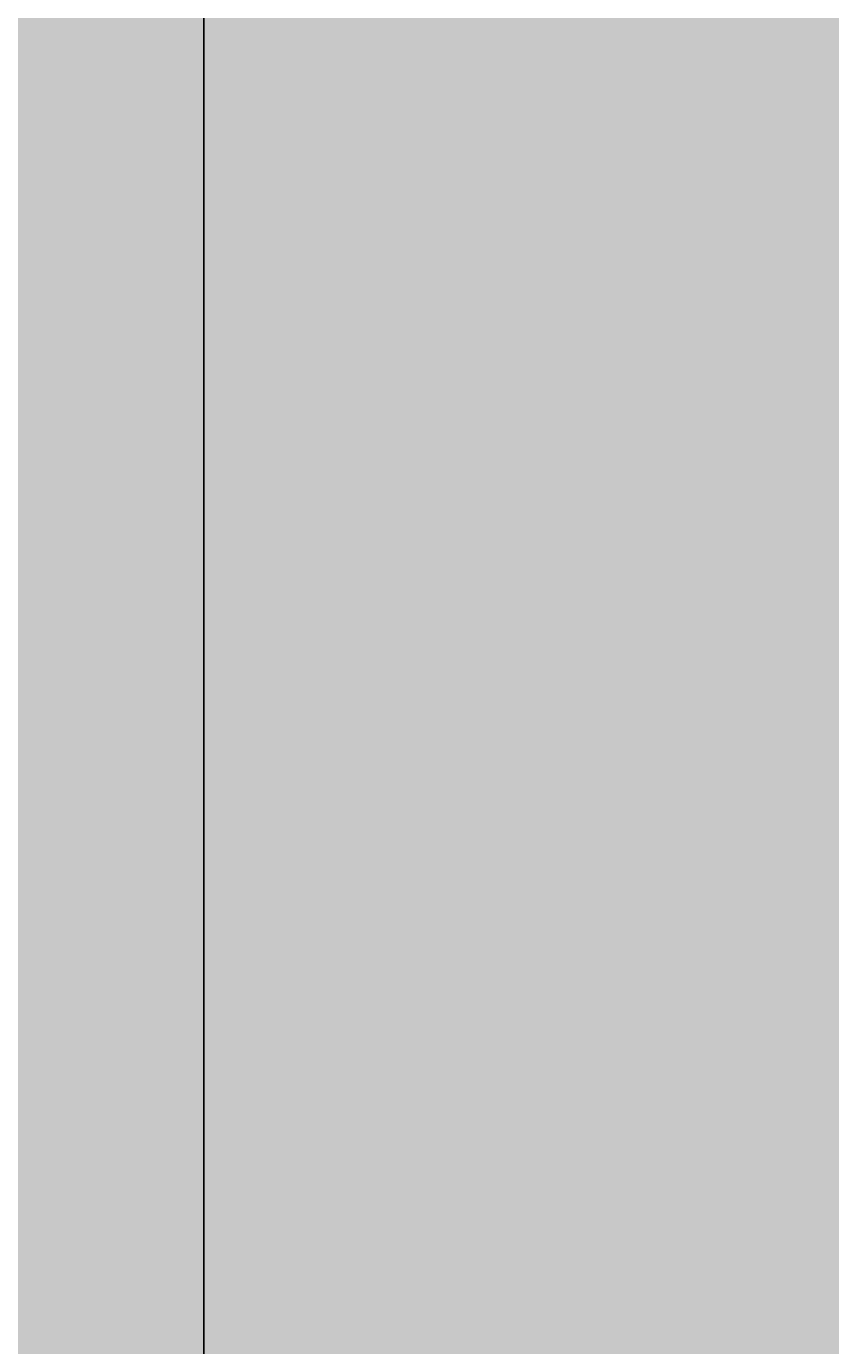
# Model space of a CAD drawing. Units: millimetres. Extents: x -22994 to 29398, y -19990 to 20176.
# Tile 105 of 135: x 198 to 216, y 95 to 124. Entities that reach past the tile are written whole.
import ezdxf

# ---------------------------------------------------------------- set-up
doc = ezdxf.new("R2010")
doc.units = ezdxf.units.MM
doc.header["$MEASUREMENT"] = 0
for name, color, linetype, lineweight in [('M-DIMS', 2, 'Continuous', 18), ('M-EQPM', 7, 'Continuous', 25), ('M-EQPM-PATT', 7, 'Continuous', 18)]:
    doc.layers.add(name, color=color, linetype=linetype, lineweight=lineweight)
doc.styles.get("Standard").update_dxf_attribs({"font": 'arial.ttf'})
doc.dimstyles.get("Standard").update_dxf_attribs({"dimtxt": 0.18, "dimasz": 10000, "dimexe": 0.18, "dimexo": 0.0625, "dimgap": 0.09, "dimtad": 0, "dimtih": 1, "dimtoh": 1, "dimdec": 0, "dimzin": 0, "dimdsep": 46, "dimtxsty": 'Standard', "dimcen": 0.09, "dimadec": 0, "dimazin": 0, "dimtfac": 1, "dimtdec": 0, "dimtofl": 0, "dimtmove": 0, "dimatfit": 3, "dimfxl": 1, "dimtolj": 1, "dimtzin": 0, "dimlwd": 30, "dimarcsym": 0})

# ---------------------------------------------------------------- blocks, each defined once
blk = doc.blocks.new('*D2')
at = {"layer": 'Defpoints', "color": 0, "transparency": 16777216}
for p in [(6.677, 10.271), (290.852, 10.271), (290.852, -5.079)]:
    blk.add_point(p, dxfattribs=at)
at = {"layer": 'M-DIMS', "color": 0, "lineweight": -2, "transparency": 16777216}
for p, q in [((6.677, 10.209), (6.677, -5.259)), ((290.852, 10.209), (290.852, -5.259))]:
    blk.add_line(p, q, dxfattribs=at)
at = {"layer": 'M-DIMS', "color": 0, "lineweight": 30, "transparency": 16777216}
for p, q in [((-9993.323, -5.079), (-19993.323, -5.079)), ((10290.852, -5.079), (20290.852, -5.079))]:
    blk.add_line(p, q, dxfattribs=at)
at = {"layer": 'M-DIMS', "color": 0, "transparency": 16777216}
for points in [[(-9993.323, 1661.588), (-9993.323, -1671.745), (6.677, -5.079)], [(10290.852, 1661.588), (10290.852, -1671.745), (290.852, -5.079)]]:
    blk.add_solid(points, dxfattribs=at)
at = {"layer": 'M-DIMS', "color": 0, "transparency": 16777216, "insert": (148.765, -5.079), "char_height": 0.18, "attachment_point": 5}
blk.add_mtext('\\A1;284.2', dxfattribs=at)
blk = doc.blocks.new('*D3')
at = {"layer": 'Defpoints', "color": 0, "transparency": 16777216}
for p in [(110.265, 204.165), (110.265, 176.366), (95.833, 127.967)]:
    blk.add_point(p, dxfattribs=at)
at = {"layer": 'M-DIMS', "color": 0, "lineweight": -2, "transparency": 16777216}
for p, q in [((95.833, 128.03), (95.833, 204.345)), ((110.265, 176.429), (110.265, 204.345))]:
    blk.add_line(p, q, dxfattribs=at)
at = {"layer": 'M-DIMS', "color": 0, "lineweight": 30, "transparency": 16777216}
for p, q in [((-9904.167, 204.165), (-19904.167, 204.165)), ((10110.265, 204.165), (20110.265, 204.165))]:
    blk.add_line(p, q, dxfattribs=at)
at = {"layer": 'M-DIMS', "color": 0, "transparency": 16777216}
for points in [[(-9904.167, 1870.832), (-9904.167, -1462.501), (95.833, 204.165)], [(10110.265, 1870.832), (10110.265, -1462.501), (110.265, 204.165)]]:
    blk.add_solid(points, dxfattribs=at)
at = {"layer": 'M-DIMS', "color": 0, "transparency": 16777216, "insert": (103.049, 204.165), "char_height": 0.18, "attachment_point": 5}
blk.add_mtext('\\A1;14.432', dxfattribs=at)
blk = doc.blocks.new('*D4')
at = {"layer": 'Defpoints', "color": 0, "transparency": 16777216}
for p in [(116.265, 204.165), (110.265, 176.366), (116.265, 176.366)]:
    blk.add_point(p, dxfattribs=at)
at = {"layer": 'M-DIMS', "color": 0, "lineweight": -2, "transparency": 16777216}
for p, q in [((110.265, 176.429), (110.265, 204.345)), ((116.265, 176.429), (116.265, 204.345))]:
    blk.add_line(p, q, dxfattribs=at)
at = {"layer": 'M-DIMS', "color": 0, "lineweight": 30, "transparency": 16777216}
for p, q in [((-9889.735, 204.165), (-19889.735, 204.165)), ((10116.265, 204.165), (20116.265, 204.165))]:
    blk.add_line(p, q, dxfattribs=at)
at = {"layer": 'M-DIMS', "color": 0, "transparency": 16777216}
for points in [[(-9889.735, 1870.832), (-9889.735, -1462.501), (110.265, 204.165)], [(10116.265, 1870.832), (10116.265, -1462.501), (116.265, 204.165)]]:
    blk.add_solid(points, dxfattribs=at)
at = {"layer": 'M-DIMS', "color": 0, "transparency": 16777216, "insert": (113.265, 204.165), "char_height": 0.18, "attachment_point": 5}
blk.add_mtext('\\A1;6', dxfattribs=at)
blk = doc.blocks.new('*D5')
at = {"layer": 'Defpoints', "color": 0, "transparency": 16777216}
for p in [(181.265, 204.165), (116.265, 176.366), (181.265, 176.366)]:
    blk.add_point(p, dxfattribs=at)
at = {"layer": 'M-DIMS', "color": 0, "lineweight": -2, "transparency": 16777216}
for p, q in [((116.265, 176.429), (116.265, 204.345)), ((181.265, 176.429), (181.265, 204.345))]:
    blk.add_line(p, q, dxfattribs=at)
at = {"layer": 'M-DIMS', "color": 0, "lineweight": 30, "transparency": 16777216}
for p, q in [((-9883.735, 204.165), (-19883.735, 204.165)), ((10181.265, 204.165), (20181.265, 204.165))]:
    blk.add_line(p, q, dxfattribs=at)
at = {"layer": 'M-DIMS', "color": 0, "transparency": 16777216}
for points in [[(-9883.735, 1870.832), (-9883.735, -1462.501), (116.265, 204.165)], [(10181.265, 1870.832), (10181.265, -1462.501), (181.265, 204.165)]]:
    blk.add_solid(points, dxfattribs=at)
at = {"layer": 'M-DIMS', "color": 0, "transparency": 16777216, "insert": (148.765, 204.165), "char_height": 0.18, "attachment_point": 5}
blk.add_mtext('\\A1;65', dxfattribs=at)
blk = doc.blocks.new('*D6')
at = {"layer": 'Defpoints', "color": 0, "transparency": 16777216}
for p in [(187.265, 204.165), (181.265, 176.366), (187.265, 176.366)]:
    blk.add_point(p, dxfattribs=at)
at = {"layer": 'M-DIMS', "color": 0, "lineweight": -2, "transparency": 16777216}
for p, q in [((181.265, 176.429), (181.265, 204.345)), ((187.265, 176.429), (187.265, 204.345))]:
    blk.add_line(p, q, dxfattribs=at)
at = {"layer": 'M-DIMS', "color": 0, "lineweight": 30, "transparency": 16777216}
for p, q in [((-9818.735, 204.165), (-19818.735, 204.165)), ((10187.265, 204.165), (20187.265, 204.165))]:
    blk.add_line(p, q, dxfattribs=at)
at = {"layer": 'M-DIMS', "color": 0, "transparency": 16777216}
for points in [[(-9818.735, 1870.832), (-9818.735, -1462.501), (181.265, 204.165)], [(10187.265, 1870.832), (10187.265, -1462.501), (187.265, 204.165)]]:
    blk.add_solid(points, dxfattribs=at)
at = {"layer": 'M-DIMS', "color": 0, "transparency": 16777216, "insert": (184.265, 204.165), "char_height": 0.18, "attachment_point": 5}
blk.add_mtext('\\A1;6', dxfattribs=at)
blk = doc.blocks.new('*D7')
at = {"layer": 'Defpoints', "color": 0, "transparency": 16777216}
for p in [(201.697, 204.165), (187.265, 176.366), (201.697, 127.967)]:
    blk.add_point(p, dxfattribs=at)
at = {"layer": 'M-DIMS', "color": 0, "lineweight": -2, "transparency": 16777216}
for p, q in [((187.265, 176.429), (187.265, 204.345)), ((201.697, 128.03), (201.697, 204.345))]:
    blk.add_line(p, q, dxfattribs=at)
at = {"layer": 'M-DIMS', "color": 0, "lineweight": 30, "transparency": 16777216}
for p, q in [((-9812.735, 204.165), (-19812.735, 204.165)), ((10201.697, 204.165), (20201.697, 204.165))]:
    blk.add_line(p, q, dxfattribs=at)
at = {"layer": 'M-DIMS', "color": 0, "transparency": 16777216}
for points in [[(-9812.735, 1870.832), (-9812.735, -1462.501), (187.265, 204.165)], [(10201.697, 1870.832), (10201.697, -1462.501), (201.697, 204.165)]]:
    blk.add_solid(points, dxfattribs=at)
at = {"layer": 'M-DIMS', "color": 0, "transparency": 16777216, "insert": (194.481, 204.165), "char_height": 0.18, "attachment_point": 5}
blk.add_mtext('\\A1;14.432', dxfattribs=at)
blk = doc.blocks.new('*D8')
at = {"layer": 'Defpoints', "color": 0, "transparency": 16777216}
for p in [(227.648, 204.165), (227.648, 146.73), (201.697, 127.967)]:
    blk.add_point(p, dxfattribs=at)
at = {"layer": 'M-DIMS', "color": 0, "lineweight": -2, "transparency": 16777216}
for p, q in [((201.697, 128.03), (201.697, 204.345)), ((227.648, 146.792), (227.648, 204.345))]:
    blk.add_line(p, q, dxfattribs=at)
at = {"layer": 'M-DIMS', "color": 0, "lineweight": 30, "transparency": 16777216}
for p, q in [((-9798.303, 204.165), (-19798.303, 204.165)), ((10227.648, 204.165), (20227.648, 204.165))]:
    blk.add_line(p, q, dxfattribs=at)
at = {"layer": 'M-DIMS', "color": 0, "transparency": 16777216}
for points in [[(-9798.303, 1870.832), (-9798.303, -1462.501), (201.697, 204.165)], [(10227.648, 1870.832), (10227.648, -1462.501), (227.648, 204.165)]]:
    blk.add_solid(points, dxfattribs=at)
at = {"layer": 'M-DIMS', "color": 0, "transparency": 16777216, "insert": (214.673, 204.165), "char_height": 0.18, "attachment_point": 5}
blk.add_mtext('\\A1;25.95', dxfattribs=at)
blk = doc.blocks.new('*D9')
at = {"layer": 'Defpoints', "color": 0, "transparency": 16777216}
for p in [(187.265, 176.366), (306.202, 176.366), (290.852, 10.271)]:
    blk.add_point(p, dxfattribs=at)
at = {"layer": 'M-DIMS', "color": 0, "lineweight": 30, "transparency": 16777216}
for p, q in [((306.202, 10176.366), (306.202, 20176.366)), ((306.202, -9989.729), (306.202, -19989.729))]:
    blk.add_line(p, q, dxfattribs=at)
at = {"layer": 'M-DIMS', "color": 0, "lineweight": -2, "transparency": 16777216}
for p, q in [((187.327, 176.366), (306.382, 176.366)), ((290.915, 10.271), (306.382, 10.271))]:
    blk.add_line(p, q, dxfattribs=at)
at = {"layer": 'M-DIMS', "color": 0, "transparency": 16777216}
for points in [[(-1360.465, 10176.366), (1972.869, 10176.366), (306.202, 176.366)], [(-1360.465, -9989.729), (1972.869, -9989.729), (306.202, 10.271)]]:
    blk.add_solid(points, dxfattribs=at)
at = {"layer": 'M-DIMS', "color": 0, "transparency": 16777216, "insert": (306.202, 93.319), "char_height": 0.18, "attachment_point": 5}
blk.add_mtext('\\A1;166.1', dxfattribs=at)
blk = doc.blocks.new('*D10')
at = {"layer": 'Defpoints', "color": 0, "transparency": 16777216}
for p in [(125.65, 136.071), (133.346, 136.071), (133.346, -5.079)]:
    blk.add_point(p, dxfattribs=at)
at = {"layer": 'M-DIMS', "color": 0, "lineweight": -2, "transparency": 16777216}
for p, q in [((125.65, 136.009), (125.65, -5.259)), ((133.346, 136.009), (133.346, -5.259))]:
    blk.add_line(p, q, dxfattribs=at)
at = {"layer": 'M-DIMS', "color": 0, "lineweight": 30, "transparency": 16777216}
for p, q in [((-9874.35, -5.079), (-19874.35, -5.079)), ((10133.346, -5.079), (20133.346, -5.079))]:
    blk.add_line(p, q, dxfattribs=at)
at = {"layer": 'M-DIMS', "color": 0, "transparency": 16777216}
for points in [[(-9874.35, 1661.588), (-9874.35, -1671.745), (125.65, -5.079)], [(10133.346, 1661.588), (10133.346, -1671.745), (133.346, -5.079)]]:
    blk.add_solid(points, dxfattribs=at)
at = {"layer": 'M-DIMS', "color": 0, "transparency": 16777216, "insert": (129.498, -5.079), "char_height": 0.18, "attachment_point": 5}
blk.add_mtext('\\A1;7.696', dxfattribs=at)
blk = doc.blocks.new('*D11')
at = {"layer": 'Defpoints', "color": 0, "transparency": 16777216}
for p in [(133.346, 136.071), (135.65, 136.071), (135.65, -5.079)]:
    blk.add_point(p, dxfattribs=at)
at = {"layer": 'M-DIMS', "color": 0, "lineweight": -2, "transparency": 16777216}
for p, q in [((133.346, 136.009), (133.346, -5.259)), ((135.65, 136.009), (135.65, -5.259))]:
    blk.add_line(p, q, dxfattribs=at)
at = {"layer": 'M-DIMS', "color": 0, "lineweight": 30, "transparency": 16777216}
for p, q in [((-9866.654, -5.079), (-19866.654, -5.079)), ((10135.65, -5.079), (20135.65, -5.079))]:
    blk.add_line(p, q, dxfattribs=at)
at = {"layer": 'M-DIMS', "color": 0, "transparency": 16777216}
for points in [[(-9866.654, 1661.588), (-9866.654, -1671.745), (133.346, -5.079)], [(10135.65, 1661.588), (10135.65, -1671.745), (135.65, -5.079)]]:
    blk.add_solid(points, dxfattribs=at)
at = {"layer": 'M-DIMS', "color": 0, "transparency": 16777216, "insert": (134.498, -5.079), "char_height": 0.18, "attachment_point": 5}
blk.add_mtext('\\A1;2.304', dxfattribs=at)
blk = doc.blocks.new('*D12')
at = {"layer": 'Defpoints', "color": 0, "transparency": 16777216}
for p in [(135.65, 136.071), (145.65, 136.071), (145.65, -5.079)]:
    blk.add_point(p, dxfattribs=at)
at = {"layer": 'M-DIMS', "color": 0, "lineweight": -2, "transparency": 16777216}
for p, q in [((135.65, 136.009), (135.65, -5.259)), ((145.65, 136.009), (145.65, -5.259))]:
    blk.add_line(p, q, dxfattribs=at)
at = {"layer": 'M-DIMS', "color": 0, "lineweight": 30, "transparency": 16777216}
for p, q in [((-9864.35, -5.079), (-19864.35, -5.079)), ((10145.65, -5.079), (20145.65, -5.079))]:
    blk.add_line(p, q, dxfattribs=at)
at = {"layer": 'M-DIMS', "color": 0, "transparency": 16777216}
for points in [[(-9864.35, 1661.588), (-9864.35, -1671.745), (135.65, -5.079)], [(10145.65, 1661.588), (10145.65, -1671.745), (145.65, -5.079)]]:
    blk.add_solid(points, dxfattribs=at)
at = {"layer": 'M-DIMS', "color": 0, "transparency": 16777216, "insert": (140.65, -5.079), "char_height": 0.18, "attachment_point": 5}
blk.add_mtext('\\A1;10', dxfattribs=at)
blk = doc.blocks.new('*D13')
at = {"layer": 'Defpoints', "color": 0, "transparency": 16777216}
for p in [(145.65, 136.071), (155.65, 136.071), (155.65, -5.079)]:
    blk.add_point(p, dxfattribs=at)
at = {"layer": 'M-DIMS', "color": 0, "lineweight": -2, "transparency": 16777216}
for p, q in [((145.65, 136.009), (145.65, -5.259)), ((155.65, 136.009), (155.65, -5.259))]:
    blk.add_line(p, q, dxfattribs=at)
at = {"layer": 'M-DIMS', "color": 0, "lineweight": 30, "transparency": 16777216}
for p, q in [((-9854.35, -5.079), (-19854.35, -5.079)), ((10155.65, -5.079), (20155.65, -5.079))]:
    blk.add_line(p, q, dxfattribs=at)
at = {"layer": 'M-DIMS', "color": 0, "transparency": 16777216}
for points in [[(-9854.35, 1661.588), (-9854.35, -1671.745), (145.65, -5.079)], [(10155.65, 1661.588), (10155.65, -1671.745), (155.65, -5.079)]]:
    blk.add_solid(points, dxfattribs=at)
at = {"layer": 'M-DIMS', "color": 0, "transparency": 16777216, "insert": (150.65, -5.079), "char_height": 0.18, "attachment_point": 5}
blk.add_mtext('\\A1;10', dxfattribs=at)
blk = doc.blocks.new('*D14')
at = {"layer": 'Defpoints', "color": 0, "transparency": 16777216}
for p in [(155.65, 136.071), (165.65, 136.071), (165.65, -5.079)]:
    blk.add_point(p, dxfattribs=at)
at = {"layer": 'M-DIMS', "color": 0, "lineweight": -2, "transparency": 16777216}
for p, q in [((155.65, 136.009), (155.65, -5.259)), ((165.65, 136.009), (165.65, -5.259))]:
    blk.add_line(p, q, dxfattribs=at)
at = {"layer": 'M-DIMS', "color": 0, "lineweight": 30, "transparency": 16777216}
for p, q in [((-9844.35, -5.079), (-19844.35, -5.079)), ((10165.65, -5.079), (20165.65, -5.079))]:
    blk.add_line(p, q, dxfattribs=at)
at = {"layer": 'M-DIMS', "color": 0, "transparency": 16777216}
for points in [[(-9844.35, 1661.588), (-9844.35, -1671.745), (155.65, -5.079)], [(10165.65, 1661.588), (10165.65, -1671.745), (165.65, -5.079)]]:
    blk.add_solid(points, dxfattribs=at)
at = {"layer": 'M-DIMS', "color": 0, "transparency": 16777216, "insert": (160.65, -5.079), "char_height": 0.18, "attachment_point": 5}
blk.add_mtext('\\A1;10', dxfattribs=at)
blk = doc.blocks.new('*D15')
at = {"layer": 'Defpoints', "color": 0, "transparency": 16777216}
for p in [(173.346, 154.788), (173.346, 136.071), (306.202, 136.071)]:
    blk.add_point(p, dxfattribs=at)
at = {"layer": 'M-DIMS', "color": 0, "lineweight": 30, "transparency": 16777216}
for p, q in [((306.202, 10154.788), (306.202, 20154.788)), ((306.202, -9863.929), (306.202, -19863.929))]:
    blk.add_line(p, q, dxfattribs=at)
at = {"layer": 'M-DIMS', "color": 0, "lineweight": -2, "transparency": 16777216}
for p, q in [((173.408, 154.788), (306.382, 154.788)), ((173.408, 136.071), (306.382, 136.071))]:
    blk.add_line(p, q, dxfattribs=at)
at = {"layer": 'M-DIMS', "color": 0, "transparency": 16777216}
for points in [[(-1360.465, 10154.788), (1972.869, 10154.788), (306.202, 154.788)], [(-1360.465, -9863.929), (1972.869, -9863.929), (306.202, 136.071)]]:
    blk.add_solid(points, dxfattribs=at)
at = {"layer": 'M-DIMS', "color": 0, "transparency": 16777216, "insert": (306.202, 145.43), "char_height": 0.18, "attachment_point": 5}
blk.add_mtext('\\A1;18.717', dxfattribs=at)
blk = doc.blocks.new('*D16')
at = {"layer": 'Defpoints', "color": 0, "transparency": 16777216}
for p in [(120.17, 204.165), (110.466, 48.035), (120.17, 48.035)]:
    blk.add_point(p, dxfattribs=at)
at = {"layer": 'M-DIMS', "color": 0, "lineweight": -2, "transparency": 16777216}
for p, q in [((110.466, 48.097), (110.466, 204.345)), ((120.17, 48.097), (120.17, 204.345))]:
    blk.add_line(p, q, dxfattribs=at)
at = {"layer": 'M-DIMS', "color": 0, "lineweight": 30, "transparency": 16777216}
for p, q in [((-9889.534, 204.165), (-19889.534, 204.165)), ((10120.17, 204.165), (20120.17, 204.165))]:
    blk.add_line(p, q, dxfattribs=at)
at = {"layer": 'M-DIMS', "color": 0, "transparency": 16777216}
for points in [[(-9889.534, 1870.832), (-9889.534, -1462.501), (110.466, 204.165)], [(10120.17, 1870.832), (10120.17, -1462.501), (120.17, 204.165)]]:
    blk.add_solid(points, dxfattribs=at)
at = {"layer": 'M-DIMS', "color": 0, "transparency": 16777216, "insert": (115.318, 204.165), "char_height": 0.18, "attachment_point": 5}
blk.add_mtext('\\A1;9.704', dxfattribs=at)
blk = doc.blocks.new('*D17')
at = {"layer": 'Defpoints', "color": 0, "transparency": 16777216}
for p in [(126.17, 204.165), (120.17, 48.035), (126.17, 48.035)]:
    blk.add_point(p, dxfattribs=at)
at = {"layer": 'M-DIMS', "color": 0, "lineweight": -2, "transparency": 16777216}
for p, q in [((120.17, 48.097), (120.17, 204.345)), ((126.17, 48.097), (126.17, 204.345))]:
    blk.add_line(p, q, dxfattribs=at)
at = {"layer": 'M-DIMS', "color": 0, "lineweight": 30, "transparency": 16777216}
for p, q in [((-9879.83, 204.165), (-19879.83, 204.165)), ((10126.17, 204.165), (20126.17, 204.165))]:
    blk.add_line(p, q, dxfattribs=at)
at = {"layer": 'M-DIMS', "color": 0, "transparency": 16777216}
for points in [[(-9879.83, 1870.832), (-9879.83, -1462.501), (120.17, 204.165)], [(10126.17, 1870.832), (10126.17, -1462.501), (126.17, 204.165)]]:
    blk.add_solid(points, dxfattribs=at)
at = {"layer": 'M-DIMS', "color": 0, "transparency": 16777216, "insert": (123.17, 204.165), "char_height": 0.18, "attachment_point": 5}
blk.add_mtext('\\A1;6', dxfattribs=at)
blk = doc.blocks.new('*D18')
at = {"layer": 'Defpoints', "color": 0, "transparency": 16777216}
for p in [(132.17, 204.165), (126.17, 48.035), (132.17, 48.035)]:
    blk.add_point(p, dxfattribs=at)
at = {"layer": 'M-DIMS', "color": 0, "lineweight": -2, "transparency": 16777216}
for p, q in [((126.17, 48.097), (126.17, 204.345)), ((132.17, 48.097), (132.17, 204.345))]:
    blk.add_line(p, q, dxfattribs=at)
at = {"layer": 'M-DIMS', "color": 0, "lineweight": 30, "transparency": 16777216}
for p, q in [((-9873.83, 204.165), (-19873.83, 204.165)), ((10132.17, 204.165), (20132.17, 204.165))]:
    blk.add_line(p, q, dxfattribs=at)
at = {"layer": 'M-DIMS', "color": 0, "transparency": 16777216}
for points in [[(-9873.83, 1870.832), (-9873.83, -1462.501), (126.17, 204.165)], [(10132.17, 1870.832), (10132.17, -1462.501), (132.17, 204.165)]]:
    blk.add_solid(points, dxfattribs=at)
at = {"layer": 'M-DIMS', "color": 0, "transparency": 16777216, "insert": (129.17, 204.165), "char_height": 0.18, "attachment_point": 5}
blk.add_mtext('\\A1;6', dxfattribs=at)
blk = doc.blocks.new('*D19')
at = {"layer": 'Defpoints', "color": 0, "transparency": 16777216}
for p in [(138.17, 204.165), (132.17, 48.035), (138.17, 48.035)]:
    blk.add_point(p, dxfattribs=at)
at = {"layer": 'M-DIMS', "color": 0, "lineweight": -2, "transparency": 16777216}
for p, q in [((132.17, 48.097), (132.17, 204.345)), ((138.17, 48.097), (138.17, 204.345))]:
    blk.add_line(p, q, dxfattribs=at)
at = {"layer": 'M-DIMS', "color": 0, "lineweight": 30, "transparency": 16777216}
for p, q in [((-9867.83, 204.165), (-19867.83, 204.165)), ((10138.17, 204.165), (20138.17, 204.165))]:
    blk.add_line(p, q, dxfattribs=at)
at = {"layer": 'M-DIMS', "color": 0, "transparency": 16777216}
for points in [[(-9867.83, 1870.832), (-9867.83, -1462.501), (132.17, 204.165)], [(10138.17, 1870.832), (10138.17, -1462.501), (138.17, 204.165)]]:
    blk.add_solid(points, dxfattribs=at)
at = {"layer": 'M-DIMS', "color": 0, "transparency": 16777216, "insert": (135.17, 204.165), "char_height": 0.18, "attachment_point": 5}
blk.add_mtext('\\A1;6', dxfattribs=at)
blk = doc.blocks.new('*D20')
at = {"layer": 'Defpoints', "color": 0, "transparency": 16777216}
for p in [(144.17, 204.165), (138.17, 48.035), (144.17, 48.035)]:
    blk.add_point(p, dxfattribs=at)
at = {"layer": 'M-DIMS', "color": 0, "lineweight": -2, "transparency": 16777216}
for p, q in [((138.17, 48.097), (138.17, 204.345)), ((144.17, 48.097), (144.17, 204.345))]:
    blk.add_line(p, q, dxfattribs=at)
at = {"layer": 'M-DIMS', "color": 0, "lineweight": 30, "transparency": 16777216}
for p, q in [((-9861.83, 204.165), (-19861.83, 204.165)), ((10144.17, 204.165), (20144.17, 204.165))]:
    blk.add_line(p, q, dxfattribs=at)
at = {"layer": 'M-DIMS', "color": 0, "transparency": 16777216}
for points in [[(-9861.83, 1870.832), (-9861.83, -1462.501), (138.17, 204.165)], [(10144.17, 1870.832), (10144.17, -1462.501), (144.17, 204.165)]]:
    blk.add_solid(points, dxfattribs=at)
at = {"layer": 'M-DIMS', "color": 0, "transparency": 16777216, "insert": (141.17, 204.165), "char_height": 0.18, "attachment_point": 5}
blk.add_mtext('\\A1;6', dxfattribs=at)
blk = doc.blocks.new('*D21')
at = {"layer": 'Defpoints', "color": 0, "transparency": 16777216}
for p in [(149.116, 204.165), (144.17, 48.035), (149.116, 48.035)]:
    blk.add_point(p, dxfattribs=at)
at = {"layer": 'M-DIMS', "color": 0, "lineweight": -2, "transparency": 16777216}
for p, q in [((144.17, 48.097), (144.17, 204.345)), ((149.116, 48.097), (149.116, 204.345))]:
    blk.add_line(p, q, dxfattribs=at)
at = {"layer": 'M-DIMS', "color": 0, "lineweight": 30, "transparency": 16777216}
for p, q in [((-9855.83, 204.165), (-19855.83, 204.165)), ((10149.116, 204.165), (20149.116, 204.165))]:
    blk.add_line(p, q, dxfattribs=at)
at = {"layer": 'M-DIMS', "color": 0, "transparency": 16777216}
for points in [[(-9855.83, 1870.832), (-9855.83, -1462.501), (144.17, 204.165)], [(10149.116, 1870.832), (10149.116, -1462.501), (149.116, 204.165)]]:
    blk.add_solid(points, dxfattribs=at)
at = {"layer": 'M-DIMS', "color": 0, "transparency": 16777216, "insert": (146.643, 204.165), "char_height": 0.18, "attachment_point": 5}
blk.add_mtext('\\A1;4.945', dxfattribs=at)
blk = doc.blocks.new('*D22')
at = {"layer": 'Defpoints', "color": 0, "transparency": 16777216}
for p in [(149.116, 30.99), (155.116, 30.99), (155.116, -5.079)]:
    blk.add_point(p, dxfattribs=at)
at = {"layer": 'M-DIMS', "color": 0, "lineweight": -2, "transparency": 16777216}
for p, q in [((149.116, 30.927), (149.116, -5.259)), ((155.116, 30.927), (155.116, -5.259))]:
    blk.add_line(p, q, dxfattribs=at)
at = {"layer": 'M-DIMS', "color": 0, "lineweight": 30, "transparency": 16777216}
for p, q in [((-9850.884, -5.079), (-19850.884, -5.079)), ((10155.116, -5.079), (20155.116, -5.079))]:
    blk.add_line(p, q, dxfattribs=at)
at = {"layer": 'M-DIMS', "color": 0, "transparency": 16777216}
for points in [[(-9850.884, 1661.588), (-9850.884, -1671.745), (149.116, -5.079)], [(10155.116, 1661.588), (10155.116, -1671.745), (155.116, -5.079)]]:
    blk.add_solid(points, dxfattribs=at)
at = {"layer": 'M-DIMS', "color": 0, "transparency": 16777216, "insert": (152.116, -5.079), "char_height": 0.18, "attachment_point": 5}
blk.add_mtext('\\A1;6', dxfattribs=at)
blk = doc.blocks.new('*D23')
at = {"layer": 'Defpoints', "color": 0, "transparency": 16777216}
for p in [(155.116, 30.99), (161.116, 30.99), (161.116, -5.079)]:
    blk.add_point(p, dxfattribs=at)
at = {"layer": 'M-DIMS', "color": 0, "lineweight": -2, "transparency": 16777216}
for p, q in [((155.116, 30.927), (155.116, -5.259)), ((161.116, 30.927), (161.116, -5.259))]:
    blk.add_line(p, q, dxfattribs=at)
at = {"layer": 'M-DIMS', "color": 0, "lineweight": 30, "transparency": 16777216}
for p, q in [((-9844.884, -5.079), (-19844.884, -5.079)), ((10161.116, -5.079), (20161.116, -5.079))]:
    blk.add_line(p, q, dxfattribs=at)
at = {"layer": 'M-DIMS', "color": 0, "transparency": 16777216}
for points in [[(-9844.884, 1661.588), (-9844.884, -1671.745), (155.116, -5.079)], [(10161.116, 1661.588), (10161.116, -1671.745), (161.116, -5.079)]]:
    blk.add_solid(points, dxfattribs=at)
at = {"layer": 'M-DIMS', "color": 0, "transparency": 16777216, "insert": (158.116, -5.079), "char_height": 0.18, "attachment_point": 5}
blk.add_mtext('\\A1;6', dxfattribs=at)
blk = doc.blocks.new('*D24')
at = {"layer": 'Defpoints', "color": 0, "transparency": 16777216}
for p in [(161.116, 30.99), (166.439, 30.99), (166.439, -5.079)]:
    blk.add_point(p, dxfattribs=at)
at = {"layer": 'M-DIMS', "color": 0, "lineweight": -2, "transparency": 16777216}
for p, q in [((161.116, 30.927), (161.116, -5.259)), ((166.439, 30.927), (166.439, -5.259))]:
    blk.add_line(p, q, dxfattribs=at)
at = {"layer": 'M-DIMS', "color": 0, "lineweight": 30, "transparency": 16777216}
for p, q in [((-9838.884, -5.079), (-19838.884, -5.079)), ((10166.439, -5.079), (20166.439, -5.079))]:
    blk.add_line(p, q, dxfattribs=at)
at = {"layer": 'M-DIMS', "color": 0, "transparency": 16777216}
for points in [[(-9838.884, 1661.588), (-9838.884, -1671.745), (161.116, -5.079)], [(10166.439, 1661.588), (10166.439, -1671.745), (166.439, -5.079)]]:
    blk.add_solid(points, dxfattribs=at)
at = {"layer": 'M-DIMS', "color": 0, "transparency": 16777216, "insert": (163.777, -5.079), "char_height": 0.18, "attachment_point": 5}
blk.add_mtext('\\A1;5.323', dxfattribs=at)
blk = doc.blocks.new('*D25')
at = {"layer": 'Defpoints', "color": 0, "transparency": 16777216}
for p in [(166.439, 30.99), (172.439, 30.99), (172.439, -5.079)]:
    blk.add_point(p, dxfattribs=at)
at = {"layer": 'M-DIMS', "color": 0, "lineweight": -2, "transparency": 16777216}
for p, q in [((166.439, 30.927), (166.439, -5.259)), ((172.439, 30.927), (172.439, -5.259))]:
    blk.add_line(p, q, dxfattribs=at)
at = {"layer": 'M-DIMS', "color": 0, "lineweight": 30, "transparency": 16777216}
for p, q in [((-9833.561, -5.079), (-19833.561, -5.079)), ((10172.439, -5.079), (20172.439, -5.079))]:
    blk.add_line(p, q, dxfattribs=at)
at = {"layer": 'M-DIMS', "color": 0, "transparency": 16777216}
for points in [[(-9833.561, 1661.588), (-9833.561, -1671.745), (166.439, -5.079)], [(10172.439, 1661.588), (10172.439, -1671.745), (172.439, -5.079)]]:
    blk.add_solid(points, dxfattribs=at)
at = {"layer": 'M-DIMS', "color": 0, "transparency": 16777216, "insert": (169.439, -5.079), "char_height": 0.18, "attachment_point": 5}
blk.add_mtext('\\A1;6', dxfattribs=at)
blk = doc.blocks.new('*D26')
at = {"layer": 'Defpoints', "color": 0, "transparency": 16777216}
for p in [(172.439, 30.99), (178.439, 30.99), (178.439, -5.079)]:
    blk.add_point(p, dxfattribs=at)
at = {"layer": 'M-DIMS', "color": 0, "lineweight": -2, "transparency": 16777216}
for p, q in [((172.439, 30.927), (172.439, -5.259)), ((178.439, 30.927), (178.439, -5.259))]:
    blk.add_line(p, q, dxfattribs=at)
at = {"layer": 'M-DIMS', "color": 0, "lineweight": 30, "transparency": 16777216}
for p, q in [((-9827.561, -5.079), (-19827.561, -5.079)), ((10178.439, -5.079), (20178.439, -5.079))]:
    blk.add_line(p, q, dxfattribs=at)
at = {"layer": 'M-DIMS', "color": 0, "transparency": 16777216}
for points in [[(-9827.561, 1661.588), (-9827.561, -1671.745), (172.439, -5.079)], [(10178.439, 1661.588), (10178.439, -1671.745), (178.439, -5.079)]]:
    blk.add_solid(points, dxfattribs=at)
at = {"layer": 'M-DIMS', "color": 0, "transparency": 16777216, "insert": (175.439, -5.079), "char_height": 0.18, "attachment_point": 5}
blk.add_mtext('\\A1;6', dxfattribs=at)
blk = doc.blocks.new('*D27')
at = {"layer": 'Defpoints', "color": 0, "transparency": 16777216}
for p in [(178.439, 30.99), (188.117, 30.99), (188.117, -5.079)]:
    blk.add_point(p, dxfattribs=at)
at = {"layer": 'M-DIMS', "color": 0, "lineweight": -2, "transparency": 16777216}
for p, q in [((178.439, 30.927), (178.439, -5.259)), ((188.117, 30.927), (188.117, -5.259))]:
    blk.add_line(p, q, dxfattribs=at)
at = {"layer": 'M-DIMS', "color": 0, "lineweight": 30, "transparency": 16777216}
for p, q in [((-9821.561, -5.079), (-19821.561, -5.079)), ((10188.117, -5.079), (20188.117, -5.079))]:
    blk.add_line(p, q, dxfattribs=at)
at = {"layer": 'M-DIMS', "color": 0, "transparency": 16777216}
for points in [[(-9821.561, 1661.588), (-9821.561, -1671.745), (178.439, -5.079)], [(10188.117, 1661.588), (10188.117, -1671.745), (188.117, -5.079)]]:
    blk.add_solid(points, dxfattribs=at)
at = {"layer": 'M-DIMS', "color": 0, "transparency": 16777216, "insert": (183.278, -5.079), "char_height": 0.18, "attachment_point": 5}
blk.add_mtext('\\A1;9.679', dxfattribs=at)
blk = doc.blocks.new('*D28')
at = {"layer": 'Defpoints', "color": 0, "transparency": 16777216}
for p in [(188.117, 48.035), (306.202, 48.035), (188.117, 30.99)]:
    blk.add_point(p, dxfattribs=at)
at = {"layer": 'M-DIMS', "color": 0, "lineweight": 30, "transparency": 16777216}
for p, q in [((306.202, 10048.035), (306.202, 20048.035)), ((306.202, -9969.01), (306.202, -19969.01))]:
    blk.add_line(p, q, dxfattribs=at)
at = {"layer": 'M-DIMS', "color": 0, "lineweight": -2, "transparency": 16777216}
for p, q in [((188.18, 48.035), (306.382, 48.035)), ((188.18, 30.99), (306.382, 30.99))]:
    blk.add_line(p, q, dxfattribs=at)
at = {"layer": 'M-DIMS', "color": 0, "transparency": 16777216}
for points in [[(-1360.465, 10048.035), (1972.869, 10048.035), (306.202, 48.035)], [(-1360.465, -9969.01), (1972.869, -9969.01), (306.202, 30.99)]]:
    blk.add_solid(points, dxfattribs=at)
at = {"layer": 'M-DIMS', "color": 0, "transparency": 16777216, "insert": (306.202, 39.512), "char_height": 0.18, "attachment_point": 5}
blk.add_mtext('\\A1;17.045', dxfattribs=at)
blk = doc.blocks.new('*D29')
at = {"layer": 'Defpoints', "color": 0, "transparency": 16777216}
for p in [(36.801, 80.045), (64.03, 80.045)]:
    blk.add_point(p, dxfattribs=at)
at = {"layer": 'M-DIMS', "color": 0, "lineweight": -2, "transparency": 16777216}
for p, q in [((50.325, 80.045), (50.505, 80.045)), ((50.415, 79.955), (50.415, 80.135))]:
    blk.add_line(p, q, dxfattribs=at)
at = {"layer": 'M-DIMS', "color": 0, "lineweight": 30, "transparency": 16777216}
blk.add_line((20064.03, 80.03), (10064.03, 80.038), dxfattribs=at)
at = {"layer": 'M-DIMS', "color": 0, "transparency": 16777216}
blk.add_solid([(10064.031, 1746.704), (10064.028, -1586.629), (64.03, 80.045)], dxfattribs=at)
at = {"layer": 'M-DIMS', "color": 0, "transparency": 16777216, "insert": (20064.521, 80.03), "char_height": 0.18, "attachment_point": 5}
blk.add_mtext('\\A1;∅27.23', dxfattribs=at)
blk = doc.blocks.new('*D34')
at = {"layer": 'Defpoints', "color": 0, "transparency": 16777216}
for p in [(178.58, 122.895), (176.812, 121.128)]:
    blk.add_point(p, dxfattribs=at)
at = {"layer": 'M-DIMS', "color": 0, "lineweight": 30, "transparency": 16777216}
for p, q in [((14322.436, 14263.311), (7250.508, 7193.103)), ((24322.436, 14263.311), (14322.436, 14263.311))]:
    blk.add_line(p, q, dxfattribs=at)
at = {"layer": 'M-DIMS', "color": 0, "lineweight": -2, "transparency": 16777216}
for p, q in [((176.722, 121.128), (176.902, 121.128)), ((176.812, 121.038), (176.812, 121.218))]:
    blk.add_line(p, q, dxfattribs=at)
at = {"layer": 'M-DIMS', "color": 0, "transparency": 16777216}
blk.add_solid([(6072.14, 8371.758), (8428.876, 6014.448), (178.58, 122.895)], dxfattribs=at)
at = {"layer": 'M-DIMS', "color": 0, "transparency": 16777216, "insert": (24322.97, 14263.311), "char_height": 0.18, "attachment_point": 5}
blk.add_mtext('\\A1;6X R2.5', dxfattribs=at)
blk = doc.blocks.new('*D36')
at = {"layer": 'Defpoints', "color": 0, "transparency": 16777216}
for p in [(46.39, 31.303), (46.387, 26.593)]:
    blk.add_point(p, dxfattribs=at)
at = {"layer": 'M-DIMS', "color": 0, "lineweight": 30, "transparency": 16777216}
for p, q in [((57.15, 20031.301), (51.77, 10031.302)), ((10057.15, 20031.301), (57.15, 20031.301))]:
    blk.add_line(p, q, dxfattribs=at)
at = {"layer": 'M-DIMS', "color": 0, "lineweight": -2, "transparency": 16777216}
for p, q in [((46.299, 28.948), (46.479, 28.948)), ((46.389, 28.858), (46.389, 29.038))]:
    blk.add_line(p, q, dxfattribs=at)
at = {"layer": 'M-DIMS', "color": 0, "transparency": 16777216}
blk.add_solid([(-1614.896, 10032.199), (1718.436, 10030.405), (46.39, 31.303)], dxfattribs=at)
at = {"layer": 'M-DIMS', "color": 0, "transparency": 16777216, "insert": (10057.554, 20031.301), "char_height": 0.18, "attachment_point": 5}
blk.add_mtext('\\A1;∅4.71', dxfattribs=at)
blk = doc.blocks.new('*D37')
at = {"layer": 'Defpoints', "color": 0, "transparency": 16777216}
for p in [(54.834, 118.615), (59.494, 118.614)]:
    blk.add_point(p, dxfattribs=at)
at = {"layer": 'M-DIMS', "color": 0, "lineweight": -2, "transparency": 16777216}
for p, q in [((57.074, 118.614), (57.254, 118.614)), ((57.164, 118.524), (57.164, 118.704))]:
    blk.add_line(p, q, dxfattribs=at)
at = {"layer": 'M-DIMS', "color": 0, "lineweight": 30, "transparency": 16777216}
blk.add_line((20059.493, 116.253), (10059.494, 117.434), dxfattribs=at)
at = {"layer": 'M-DIMS', "color": 0, "transparency": 16777216}
blk.add_solid([(10059.69, 1784.1), (10059.297, -1549.233), (59.494, 118.614)], dxfattribs=at)
at = {"layer": 'M-DIMS', "color": 0, "transparency": 16777216, "insert": (20059.985, 116.253), "char_height": 0.18, "attachment_point": 5}
blk.add_mtext('\\A1;∅4.659', dxfattribs=at)

msp = doc.modelspace()

# ---------------------------------------------------------------- hatches: boundary and pattern name
at = {"layer": 'M-EQPM-PATT'}
h = msp.add_hatch(color=256, dxfattribs=at)
h.set_gradient(color1=(205, 32, 39), color2=(205, 32, 39), tint=1)
h.paths.add_polyline_path([(116.2647, 150.3662), (116.2647, 170.3662), (116.2647, 176.3662), (110.2647, 176.3662), (110.2647, 152.0276), (95.8327, 127.967), (95.8327, 16.6063), (201.6967, 16.6063), (201.6967, 127.967), (187.2647, 152.0276), (187.2647, 176.3662), (181.2647, 176.3662), (181.2647, 170.3662), (181.2647, 150.3662), (195.6967, 126.3055), (195.6967, 22.6063), (101.8327, 22.6063), (101.8327, 126.3055)])
h.paths.add_polyline_path([(185.2208, 88.6347), (101.8327, 88.6347), (101.8327, 87.6347), (182.8066, 87.6347), (178.7313, 83.5594), (195.6967, 83.5594), (195.6967, 84.5594), (181.1455, 84.5594)], flags=17)
h.paths.add_polyline_path([(95.8327, 88.6347), (60.9779, 88.6347, -0.0228552), (61.7178, 87.6347), (95.8327, 87.6347)])
h.paths.add_polyline_path([(215.6212, 86.5189), (215.6212, 80.5999), (220.5095, 83.5594)])
h.paths.add_polyline_path([(215.6212, 84.5594), (201.6967, 84.5594), (201.6967, 83.5594), (215.6212, 83.5594)])
h.paths.add_polyline_path([(225.3978, 86.5189), (220.5095, 83.5594), (225.3978, 80.5999)])
h.paths.add_polyline_path([(231.6256, 84.5594), (225.3978, 84.5594), (225.3978, 83.5594), (231.6256, 83.5594)])

# ---------------------------------------------------------------- linework, layer by layer
at = {"layer": 'M-EQPM'}
msp.add_lwpolyline([(110.2647, 176.3662), (110.2647, 152.0276), (95.8327, 127.967), (95.8327, 16.6063), (201.6967, 16.6063), (201.6967, 127.967), (187.2647, 152.0276), (187.2647, 176.3662)], close=True, dxfattribs=at)

# ---------------------------------------------------------------- dimensions: what is measured, and where the dimension line sits
at = {"layer": 'M-DIMS'}
for base, p1, p2, override, picture, middle in [((306.202, 176.3662), (290.852, 10.2713), (187.2647, 176.3662), {"dimdec": 1, "dimlfac": 1, "dimrnd": 0, "dimzin": 0, "dimdsep": 46, "dimlunit": 2}, '*D9', (306.202, 93.3187)), ((306.202, 136.0713), (173.3459, 154.788), (173.3459, 136.0713), {"dimdec": 3, "dimlfac": 1, "dimrnd": 0, "dimzin": 0, "dimdsep": 46, "dimlunit": 2}, '*D15', (306.202, 145.4297)), ((306.202, 48.0349), (188.1175, 30.9895), (188.1175, 48.0349), {"dimdec": 3, "dimlfac": 1, "dimrnd": 0, "dimzin": 0, "dimdsep": 46, "dimlunit": 2}, '*D28', (306.202, 39.5122))]:
    dim = msp.add_linear_dim(base=base, p1=p1, p2=p2, angle=90, dimstyle='Standard', override=override, dxfattribs=at)
    dim.commit()
    dim.dimension.update_dxf_attribs({"geometry": picture, "text_midpoint": middle})
dim = msp.add_diameter_dim_2p(p1=(46.3875, 26.5934), p2=(46.39, 31.3035), dimstyle='Standard', override={"dimdec": 2, "dimlfac": 1, "dimrnd": 0, "dimzin": 0, "dimdsep": 46, "dimlunit": 2}, dxfattribs=at)
dim.commit()
dim.dimension.update_dxf_attribs({"geometry": '*D36', "text_midpoint": (10057.5542, 20031.3006), "dimtype": 163})
dim = msp.add_radius_dim(center=(176.8123, 121.1277), mpoint=(178.5802, 122.8952), text='6X <>', dimstyle='Standard', override={"dimdec": 1, "dimlfac": 1, "dimrnd": 0, "dimzin": 0, "dimdsep": 46, "dimlunit": 2}, dxfattribs=at)
dim.commit()
dim.dimension.update_dxf_attribs({"geometry": '*D34', "text_midpoint": (24322.9703, 14263.3108)})
for base, p1, p2, override, picture, middle in [((110.2647, 204.1654), (95.8327, 127.967), (110.2647, 176.3662), {"dimdec": 3, "dimlfac": 1, "dimrnd": 0, "dimzin": 0, "dimdsep": 46, "dimlunit": 2}, '*D3', (103.0487, 204.1654)), ((116.2647, 204.1654), (110.2647, 176.3662), (116.2647, 176.3662), {"dimdec": 0, "dimlfac": 1, "dimrnd": 0, "dimzin": 0, "dimdsep": 46, "dimlunit": 2}, '*D4', (113.2647, 204.1654)), ((120.1702, 204.1654), (110.4658, 48.0349), (120.1702, 48.0349), {"dimdec": 3, "dimlfac": 1, "dimrnd": 0, "dimzin": 0, "dimdsep": 46, "dimlunit": 2}, '*D16', (115.318, 204.1654)), ((181.2647, 204.1654), (116.2647, 176.3662), (181.2647, 176.3662), {"dimdec": 0, "dimlfac": 1, "dimrnd": 0, "dimzin": 0, "dimdsep": 46, "dimlunit": 2}, '*D5', (148.7647, 204.1654)), ((126.1702, 204.1654), (120.1702, 48.0349), (126.1702, 48.0349), {"dimdec": 0, "dimlfac": 1, "dimrnd": 0, "dimzin": 0, "dimdsep": 46, "dimlunit": 2}, '*D17', (123.1702, 204.1654)), ((132.1702, 204.1654), (126.1702, 48.0349), (132.1702, 48.0349), {"dimdec": 0, "dimlfac": 1, "dimrnd": 0, "dimzin": 0, "dimdsep": 46, "dimlunit": 2}, '*D18', (129.1702, 204.1654)), ((138.1702, 204.1654), (132.1702, 48.0349), (138.1702, 48.0349), {"dimdec": 0, "dimlfac": 1, "dimrnd": 0, "dimzin": 0, "dimdsep": 46, "dimlunit": 2}, '*D19', (135.1702, 204.1654)), ((144.1702, 204.1654), (138.1702, 48.0349), (144.1702, 48.0349), {"dimdec": 0, "dimlfac": 1, "dimrnd": 0, "dimzin": 0, "dimdsep": 46, "dimlunit": 2}, '*D20', (141.1702, 204.1654)), ((149.11567, 204.16539), (144.17023, 48.03494), (149.11567, 48.03494), {"dimdec": 3, "dimlfac": 1, "dimrnd": 0, "dimzin": 0, "dimdsep": 46, "dimlunit": 2}, '*D21', (146.64295, 204.16539)), ((187.2647, 204.1654), (181.2647, 176.3662), (187.2647, 176.3662), {"dimdec": 0, "dimlfac": 1, "dimrnd": 0, "dimzin": 0, "dimdsep": 46, "dimlunit": 2}, '*D6', (184.2647, 204.1654)), ((201.6967, 204.1654), (187.2647, 176.3662), (201.6967, 127.967), {"dimdec": 3, "dimlfac": 1, "dimrnd": 0, "dimzin": 0, "dimdsep": 46, "dimlunit": 2}, '*D7', (194.4807, 204.1654)), ((227.6485, 204.1654), (201.6967, 127.967), (227.6485, 146.7296), {"dimdec": 2, "dimlfac": 1, "dimrnd": 0, "dimzin": 0, "dimdsep": 46, "dimlunit": 2}, '*D8', (214.6726, 204.1654)), ((290.852, -5.0787), (6.6773, 10.2713), (290.852, 10.2713), {"dimdec": 1, "dimlfac": 1, "dimrnd": 0, "dimzin": 0, "dimdsep": 46, "dimlunit": 2}, '*D2', (148.7647, -5.0787)), ((133.3459, -5.0787), (125.6498, 136.0713), (133.3459, 136.0713), {"dimdec": 3, "dimlfac": 1, "dimrnd": 0, "dimzin": 0, "dimdsep": 46, "dimlunit": 2}, '*D10', (129.4978, -5.0787)), ((135.6498, -5.0787), (133.3459, 136.0713), (135.6498, 136.0713), {"dimdec": 3, "dimlfac": 1, "dimrnd": 0, "dimzin": 0, "dimdsep": 46, "dimlunit": 2}, '*D11', (134.4978, -5.0787)), ((145.6498, -5.0787), (135.6498, 136.0713), (145.6498, 136.0713), {"dimdec": 0, "dimlfac": 1, "dimrnd": 0, "dimzin": 0, "dimdsep": 46, "dimlunit": 2}, '*D12', (140.6498, -5.0787)), ((155.6498, -5.0787), (145.6498, 136.0713), (155.6498, 136.0713), {"dimdec": 0, "dimlfac": 1, "dimrnd": 0, "dimzin": 0, "dimdsep": 46, "dimlunit": 2}, '*D13', (150.6498, -5.0787)), ((155.1157, -5.0787), (149.1157, 30.9895), (155.1157, 30.9895), {"dimdec": 0, "dimlfac": 1, "dimrnd": 0, "dimzin": 0, "dimdsep": 46, "dimlunit": 2}, '*D22', (152.1157, -5.0787)), ((161.1157, -5.0787), (155.1157, 30.9895), (161.1157, 30.9895), {"dimdec": 0, "dimlfac": 1, "dimrnd": 0, "dimzin": 0, "dimdsep": 46, "dimlunit": 2}, '*D23', (158.1157, -5.0787)), ((165.6498, -5.0787), (155.6498, 136.0713), (165.6498, 136.0713), {"dimdec": 0, "dimlfac": 1, "dimrnd": 0, "dimzin": 0, "dimdsep": 46, "dimlunit": 2}, '*D14', (160.6498, -5.0787)), ((166.4387, -5.0787), (161.1157, 30.9895), (166.4387, 30.9895), {"dimdec": 3, "dimlfac": 1, "dimrnd": 0, "dimzin": 0, "dimdsep": 46, "dimlunit": 2}, '*D24', (163.7772, -5.0787)), ((172.4387, -5.0787), (166.4387, 30.9895), (172.4387, 30.9895), {"dimdec": 0, "dimlfac": 1, "dimrnd": 0, "dimzin": 0, "dimdsep": 46, "dimlunit": 2}, '*D25', (169.4387, -5.0787)), ((178.4387, -5.0787), (172.4387, 30.9895), (178.4387, 30.9895), {"dimdec": 0, "dimlfac": 1, "dimrnd": 0, "dimzin": 0, "dimdsep": 46, "dimlunit": 2}, '*D26', (175.4387, -5.0787)), ((188.1175, -5.0787), (178.4387, 30.9895), (188.1175, 30.9895), {"dimdec": 3, "dimlfac": 1, "dimrnd": 0, "dimzin": 0, "dimdsep": 46, "dimlunit": 2}, '*D27', (183.2781, -5.0787))]:
    dim = msp.add_linear_dim(base=base, p1=p1, p2=p2, dimstyle='Standard', override=override, dxfattribs=at)
    dim.commit()
    dim.dimension.update_dxf_attribs({"geometry": picture, "text_midpoint": middle})
for p1, p2, override, picture, middle in [((54.8343, 118.6145), (59.4936, 118.614), {"dimdec": 3, "dimlfac": 1, "dimrnd": 0, "dimzin": 0, "dimdsep": 46, "dimlunit": 2}, '*D37', (20059.4934, 116.2531)), ((36.8006, 80.045), (64.0296, 80.045), {"dimdec": 2, "dimlfac": 1, "dimrnd": 0, "dimzin": 0, "dimdsep": 46, "dimlunit": 2}, '*D29', (20064.0296, 80.0303))]:
    dim = msp.add_diameter_dim_2p(p1=p1, p2=p2, dimstyle='Standard', override=override, dxfattribs=at)
    dim.commit()
    dim.dimension.update_dxf_attribs({"geometry": picture, "text_midpoint": middle})

doc.saveas('drawing.dxf')
